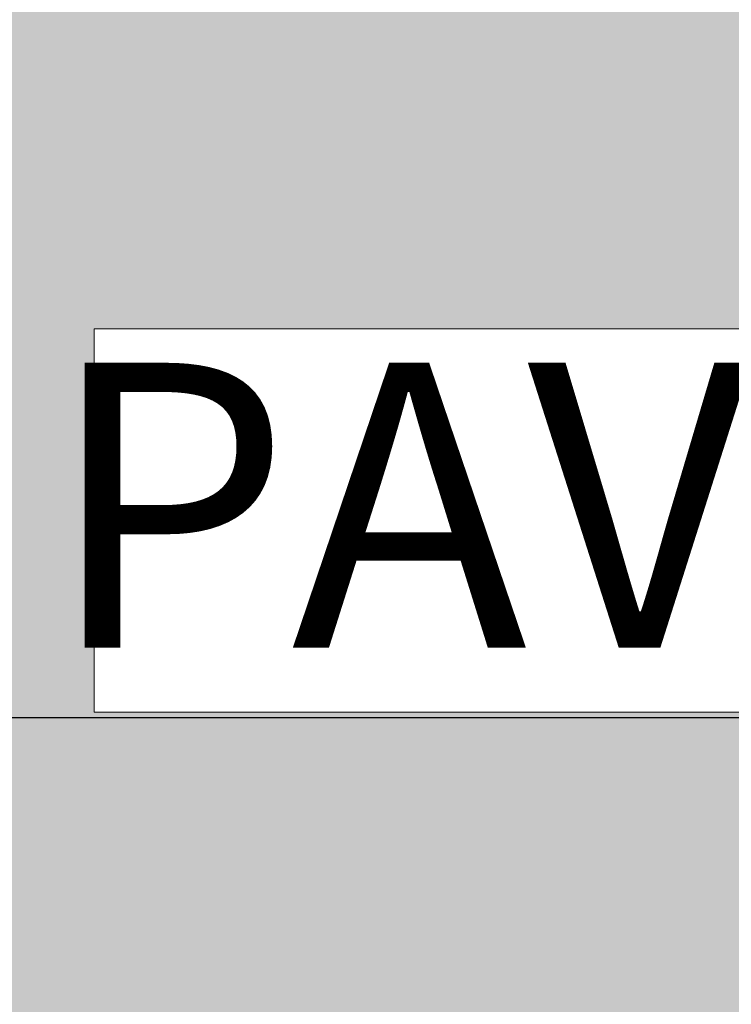
# Model space of a CAD drawing. Units: inches. Extents: x 459864 to 460310, y 324185 to 324787.
# Tile 42 of 112: x 460079 to 460094, y 324221 to 324242. Entities that reach past the tile are written whole.
import ezdxf

# ---------------------------------------------------------------- set-up
doc = ezdxf.new("R2010")
doc.units = ezdxf.units.IN
for name, color, linetype, lineweight in [('A-ANNO-DIMS', 2, 'Continuous', 18), ('L-HRDS', 9, 'Continuous', 18), ('L-SITE-PATT', 252, 'Continuous', 13)]:
    doc.layers.add(name, color=color, linetype=linetype, lineweight=lineweight)
doc.styles.get("Standard").update_dxf_attribs({"font": 'arial.ttf'})
doc.dimstyles.new('ISO-25', dxfattribs={"dimtxt": 6, "dimasz": 2.5, "dimexe": 1.25, "dimexo": 0.625, "dimtad": 1, "dimdec": 1, "dimlunit": 3, "dimtxsty": 'Standard', "dimcen": 2.5, "dimadec": 0, "dimazin": 0, "dimtfac": 1, "dimtdec": 1, "dimtmove": 0, "dimatfit": 3, "dimfxl": 1, "dimarcsym": 0})

# ---------------------------------------------------------------- blocks, each defined once
blk = doc.blocks.new('*D36')
at = {"layer": 'A-ANNO-DIMS', "color": 0, "lineweight": -2, "transparency": 16777216}
for p, q in [((460063.861, 324228.483), (460063.861, 324226.056)), ((460075.876, 324228.483), (460075.876, 324226.056)), ((460066.361, 324227.306), (460073.376, 324227.306)), ((460075.876, 324227.306), (460126.021, 324227.306))]:
    blk.add_line(p, q, dxfattribs=at)
at = {"layer": 'A-ANNO-DIMS', "color": 0, "transparency": 16777216}
for points in [[(460066.361, 324227.722), (460066.361, 324226.889), (460063.861, 324227.306)], [(460073.376, 324227.722), (460073.376, 324226.889), (460075.876, 324227.306)]]:
    blk.add_solid(points, dxfattribs=at)
at = {"layer": 'Defpoints', "color": 0, "transparency": 16777216}
for p in [(460063.861, 324229.108), (460075.876, 324229.108), (460075.876, 324227.306)]:
    blk.add_point(p, dxfattribs=at)
at = {"layer": 'A-ANNO-DIMS', "color": 0, "transparency": 16777216, "insert": (460102.199, 324230.994), "char_height": 6, "attachment_point": 5}
blk.add_mtext('PAVER 1\'-0"', dxfattribs=at)

msp = doc.modelspace()

# ---------------------------------------------------------------- hatches: boundary and pattern name
at = {"layer": 'L-SITE-PATT'}
h = msp.add_hatch(dxfattribs=at)
h.set_pattern_fill('DOTS', color=256)
h.paths.add_polyline_path([(460269.804, 324283.483), (460247.115, 324283.483), (460121.929, 324283.483), (460121.929, 324252.473), (460117.429, 324252.473), (460110.124, 324252.473), (460110.124, 324243.287), (460080.83, 324243.287), (460080.83, 324252.473), (460061.115, 324252.473), (460061.115, 324251.882), (460077.909, 324251.882), (460077.909, 324199.483), (460080.83, 324199.483), (460080.83, 324207.553), (460110.124, 324207.553), (460110.124, 324199.483), (460110.813, 324199.483), (460262.115, 324199.483), (460269.804, 324199.483)], flags=17)
edge = h.paths.add_edge_path(flags=0)
edge.add_ellipse((460222.59, 324263.813), major_axis=(-8.485, 8.485), ratio=1, start_angle=405, end_angle=495, ccw=False)
edge.add_line((460214.821, 324254.66), (460214.832, 324254.666))
edge.add_ellipse((460222.59, 324263.813), major_axis=(-8.485, 8.485), ratio=1, start_angle=405, end_angle=495, ccw=False)
edge.add_line((460210.759, 324261.781), (460210.768, 324261.787))
edge.add_ellipse((460222.59, 324263.813), major_axis=(-8.485, 8.485), ratio=1, start_angle=405, end_angle=495, ccw=False)
edge.add_ellipse((460222.59, 324263.813), major_axis=(-8.485, 8.485), ratio=1, start_angle=392.754, end_angle=405, ccw=False)
edge.add_ellipse((460222.59, 324263.813), major_axis=(-8.485, 8.485), ratio=1, start_angle=380.9347, end_angle=392.754, ccw=False)
edge.add_line((460211.337, 324267.985), (460211.34, 324267.985))
edge.add_ellipse((460222.59, 324263.813), major_axis=(-8.485, 8.485), ratio=1, start_angle=380.9347, end_angle=392.754, ccw=False)
edge.add_ellipse((460222.59, 324263.813), major_axis=(-8.485, 8.485), ratio=1, start_angle=347.9015, end_angle=380.9347, ccw=False)
edge.add_ellipse((460222.59, 324263.813), major_axis=(-8.485, 8.485), ratio=1, start_angle=327.0619, end_angle=347.9015, ccw=False)
edge.add_ellipse((460222.59, 324263.813), major_axis=(-8.485, 8.485), ratio=1, start_angle=278.3246, end_angle=327.0619, ccw=False)
edge.add_line((460225.158, 324275.536), (460225.158, 324275.535))
edge.add_ellipse((460222.59, 324263.813), major_axis=(-8.485, 8.485), ratio=1, start_angle=278.3246, end_angle=327.0619, ccw=False)
edge.add_ellipse((460222.59, 324263.813), major_axis=(-8.485, 8.485), ratio=1, start_angle=260.6436, end_angle=278.3246, ccw=False)
edge.add_ellipse((460222.59, 324263.813), major_axis=(-8.485, 8.485), ratio=1, start_angle=225, end_angle=260.6436, ccw=False)
edge.add_line((460234.509, 324265.243), (460234.501, 324265.239))
edge.add_ellipse((460222.59, 324263.813), major_axis=(-8.485, 8.485), ratio=1, start_angle=225, end_angle=260.6436, ccw=False)
edge.add_ellipse((460222.59, 324263.813), major_axis=(-8.485, 8.485), ratio=1, start_angle=495, end_angle=585, ccw=False)
edge.add_line((460234.437, 324261.861), (460234.424, 324261.858))
edge.add_ellipse((460222.59, 324263.813), major_axis=(-8.485, 8.485), ratio=1, start_angle=495, end_angle=585, ccw=False)
edge.add_line((460227.95, 324253.067), (460227.946, 324253.083))
edge.add_ellipse((460222.59, 324263.813), major_axis=(-8.485, 8.485), ratio=1, start_angle=495, end_angle=585, ccw=False)
edge.add_line((460226.223, 324252.369), (460226.211, 324252.38))
edge.add_ellipse((460222.59, 324263.813), major_axis=(-8.485, 8.485), ratio=1, start_angle=495, end_angle=585, ccw=False)
h.paths.add_polyline_path([(460219.651, 324254.347), (460218.461, 324253.545), (460218.275, 324254.789), (460219.642, 324256.542), (460219.625, 324260.848), (460216.11, 324257.333), (460214.35, 324256.978), (460215.416, 324259.356), (460212.524, 324258.496), (460213.137, 324259.93), (460218.507, 324263.813), (460222.59, 324263.813), (460222.59, 324267.807), (460218.176, 324272.212), (460219.026, 324274.639), (460222.59, 324272.811), (460222.59, 324275.423), (460223.057, 324274.825), (460222.675, 324273.492), (460225.912, 324267.135), (460219.625, 324260.848)], flags=0)
edge = h.paths.add_edge_path(flags=0)
edge.add_ellipse((460194.576, 324264.046), major_axis=(-8.485, 8.485), ratio=1, start_angle=495, end_angle=585, ccw=False)
edge.add_line((460199.936, 324253.3), (460199.932, 324253.316))
edge.add_ellipse((460194.576, 324264.046), major_axis=(-8.485, 8.485), ratio=1, start_angle=495, end_angle=585, ccw=False)
edge.add_line((460198.208, 324252.603), (460198.196, 324252.613))
edge.add_ellipse((460194.576, 324264.046), major_axis=(-8.485, 8.485), ratio=1, start_angle=495, end_angle=585, ccw=False)
edge.add_ellipse((460194.576, 324264.046), major_axis=(-8.485, 8.485), ratio=1, start_angle=405, end_angle=495, ccw=False)
edge.add_line((460186.806, 324254.893), (460186.817, 324254.899))
edge.add_ellipse((460194.576, 324264.046), major_axis=(-8.485, 8.485), ratio=1, start_angle=405, end_angle=495, ccw=False)
edge.add_line((460182.744, 324262.014), (460182.753, 324262.02))
edge.add_ellipse((460194.576, 324264.046), major_axis=(-8.485, 8.485), ratio=1, start_angle=405, end_angle=495, ccw=False)
edge.add_ellipse((460194.576, 324264.046), major_axis=(-8.485, 8.485), ratio=1, start_angle=392.754, end_angle=405, ccw=False)
edge.add_ellipse((460194.576, 324264.046), major_axis=(-8.485, 8.485), ratio=1, start_angle=380.9347, end_angle=392.754, ccw=False)
edge.add_line((460183.323, 324268.218), (460183.326, 324268.218))
edge.add_ellipse((460194.576, 324264.046), major_axis=(-8.485, 8.485), ratio=1, start_angle=380.9347, end_angle=392.754, ccw=False)
edge.add_ellipse((460194.576, 324264.046), major_axis=(-8.485, 8.485), ratio=1, start_angle=347.9015, end_angle=380.9347, ccw=False)
edge.add_ellipse((460194.576, 324264.046), major_axis=(-8.485, 8.485), ratio=1, start_angle=327.0619, end_angle=347.9015, ccw=False)
edge.add_ellipse((460194.576, 324264.046), major_axis=(-8.485, 8.485), ratio=1, start_angle=278.3246, end_angle=327.0619, ccw=False)
edge.add_line((460197.144, 324275.769), (460197.143, 324275.768))
edge.add_ellipse((460194.576, 324264.046), major_axis=(-8.485, 8.485), ratio=1, start_angle=278.3246, end_angle=327.0619, ccw=False)
edge.add_ellipse((460194.576, 324264.046), major_axis=(-8.485, 8.485), ratio=1, start_angle=260.6436, end_angle=278.3246, ccw=False)
edge.add_ellipse((460194.576, 324264.046), major_axis=(-8.485, 8.485), ratio=1, start_angle=225, end_angle=260.6436, ccw=False)
edge.add_line((460206.494, 324265.476), (460206.487, 324265.473))
edge.add_ellipse((460194.576, 324264.046), major_axis=(-8.485, 8.485), ratio=1, start_angle=225, end_angle=260.6436, ccw=False)
edge.add_ellipse((460194.576, 324264.046), major_axis=(-8.485, 8.485), ratio=1, start_angle=495, end_angle=585, ccw=False)
edge.add_line((460206.422, 324262.094), (460206.409, 324262.091))
h.paths.add_polyline_path([(460191.61, 324261.081), (460191.637, 324254.58), (460190.447, 324253.778), (460190.261, 324255.023), (460191.628, 324256.775), (460191.61, 324261.081), (460188.096, 324257.566), (460186.335, 324257.211), (460187.402, 324259.589), (460184.509, 324258.729), (460185.123, 324260.163), (460190.493, 324264.046), (460194.576, 324264.046), (460194.576, 324268.04), (460190.161, 324272.446), (460191.011, 324274.872), (460194.576, 324273.044), (460194.576, 324275.657), (460195.043, 324275.058), (460194.661, 324273.725), (460197.897, 324267.368)], flags=0)
edge = h.paths.add_edge_path(flags=0)
edge.add_ellipse((460252.912, 324263.578), major_axis=(-8.485, 8.485), ratio=1, start_angle=405, end_angle=495, ccw=False)
edge.add_line((460241.081, 324261.545), (460241.089, 324261.551))
edge.add_ellipse((460252.912, 324263.578), major_axis=(-8.485, 8.485), ratio=1, start_angle=405, end_angle=495, ccw=False)
edge.add_ellipse((460252.912, 324263.578), major_axis=(-8.485, 8.485), ratio=1, start_angle=392.754, end_angle=405, ccw=False)
edge.add_ellipse((460252.912, 324263.578), major_axis=(-8.485, 8.485), ratio=1, start_angle=380.9347, end_angle=392.754, ccw=False)
edge.add_line((460241.659, 324267.749), (460241.662, 324267.749))
edge.add_ellipse((460252.912, 324263.578), major_axis=(-8.485, 8.485), ratio=1, start_angle=380.9347, end_angle=392.754, ccw=False)
edge.add_ellipse((460252.912, 324263.578), major_axis=(-8.485, 8.485), ratio=1, start_angle=347.9015, end_angle=380.9347, ccw=False)
edge.add_ellipse((460252.912, 324263.578), major_axis=(-8.485, 8.485), ratio=1, start_angle=327.0619, end_angle=347.9015, ccw=False)
edge.add_ellipse((460252.912, 324263.578), major_axis=(-8.485, 8.485), ratio=1, start_angle=278.3246, end_angle=327.0619, ccw=False)
edge.add_line((460255.48, 324275.3), (460255.479, 324275.299))
edge.add_ellipse((460252.912, 324263.578), major_axis=(-8.485, 8.485), ratio=1, start_angle=278.3246, end_angle=327.0619, ccw=False)
edge.add_ellipse((460252.912, 324263.578), major_axis=(-8.485, 8.485), ratio=1, start_angle=260.6436, end_angle=278.3246, ccw=False)
edge.add_ellipse((460252.912, 324263.578), major_axis=(-8.485, 8.485), ratio=1, start_angle=225, end_angle=260.6436, ccw=False)
edge.add_line((460264.83, 324265.007), (460264.823, 324265.004))
edge.add_ellipse((460252.912, 324263.578), major_axis=(-8.485, 8.485), ratio=1, start_angle=225, end_angle=260.6436, ccw=False)
edge.add_ellipse((460252.912, 324263.578), major_axis=(-8.485, 8.485), ratio=1, start_angle=495, end_angle=585, ccw=False)
edge.add_line((460264.758, 324261.626), (460264.745, 324261.622))
edge.add_ellipse((460252.912, 324263.578), major_axis=(-8.485, 8.485), ratio=1, start_angle=495, end_angle=585, ccw=False)
edge.add_line((460258.272, 324252.832), (460258.268, 324252.848))
edge.add_ellipse((460252.912, 324263.578), major_axis=(-8.485, 8.485), ratio=1, start_angle=495, end_angle=585, ccw=False)
edge.add_line((460256.545, 324252.134), (460256.533, 324252.144))
edge.add_ellipse((460252.912, 324263.578), major_axis=(-8.485, 8.485), ratio=1, start_angle=495, end_angle=585, ccw=False)
edge.add_ellipse((460252.912, 324263.578), major_axis=(-8.485, 8.485), ratio=1, start_angle=405, end_angle=495, ccw=False)
edge.add_line((460245.143, 324254.424), (460245.153, 324254.43))
h.paths.add_polyline_path([(460244.672, 324256.742), (460245.738, 324259.12), (460242.846, 324258.26), (460243.459, 324259.694), (460248.829, 324263.578), (460252.912, 324263.578), (460252.912, 324267.571), (460248.497, 324271.977), (460249.348, 324274.403), (460252.912, 324272.576), (460252.912, 324275.188), (460253.379, 324274.589), (460252.997, 324273.257), (460256.233, 324266.899), (460249.946, 324260.612), (460249.973, 324254.111), (460248.783, 324253.309), (460248.597, 324254.554), (460249.964, 324256.306), (460249.946, 324260.612), (460246.432, 324257.097)], flags=0)
edge = h.paths.add_edge_path(flags=0)
edge.add_ellipse((460167.439, 324262.833), major_axis=(-8.485, 8.485), ratio=1, start_angle=495, end_angle=585, ccw=False)
edge.add_line((460172.799, 324252.087), (460172.795, 324252.103))
edge.add_ellipse((460167.439, 324262.833), major_axis=(-8.485, 8.485), ratio=1, start_angle=495, end_angle=585, ccw=False)
edge.add_line((460171.071, 324251.389), (460171.059, 324251.399))
edge.add_ellipse((460167.439, 324262.833), major_axis=(-8.485, 8.485), ratio=1, start_angle=495, end_angle=585, ccw=False)
edge.add_ellipse((460167.439, 324262.833), major_axis=(-8.485, 8.485), ratio=1, start_angle=405, end_angle=495, ccw=False)
edge.add_line((460159.669, 324253.679), (460159.68, 324253.685))
edge.add_ellipse((460167.439, 324262.833), major_axis=(-8.485, 8.485), ratio=1, start_angle=405, end_angle=495, ccw=False)
edge.add_line((460155.607, 324260.8), (460155.616, 324260.806))
edge.add_ellipse((460167.439, 324262.833), major_axis=(-8.485, 8.485), ratio=1, start_angle=405, end_angle=495, ccw=False)
edge.add_ellipse((460167.439, 324262.833), major_axis=(-8.485, 8.485), ratio=1, start_angle=392.754, end_angle=405, ccw=False)
edge.add_ellipse((460167.439, 324262.833), major_axis=(-8.485, 8.485), ratio=1, start_angle=380.9347, end_angle=392.754, ccw=False)
edge.add_line((460156.185, 324267.005), (460156.189, 324267.005))
edge.add_ellipse((460167.439, 324262.833), major_axis=(-8.485, 8.485), ratio=1, start_angle=380.9347, end_angle=392.754, ccw=False)
edge.add_ellipse((460167.439, 324262.833), major_axis=(-8.485, 8.485), ratio=1, start_angle=347.9015, end_angle=380.9347, ccw=False)
edge.add_ellipse((460167.439, 324262.833), major_axis=(-8.485, 8.485), ratio=1, start_angle=327.0619, end_angle=347.9015, ccw=False)
edge.add_ellipse((460167.439, 324262.833), major_axis=(-8.485, 8.485), ratio=1, start_angle=278.3246, end_angle=327.0619, ccw=False)
edge.add_line((460170.007, 324274.556), (460170.006, 324274.554))
edge.add_ellipse((460167.439, 324262.833), major_axis=(-8.485, 8.485), ratio=1, start_angle=278.3246, end_angle=327.0619, ccw=False)
edge.add_ellipse((460167.439, 324262.833), major_axis=(-8.485, 8.485), ratio=1, start_angle=260.6436, end_angle=278.3246, ccw=False)
edge.add_ellipse((460167.439, 324262.833), major_axis=(-8.485, 8.485), ratio=1, start_angle=225, end_angle=260.6436, ccw=False)
edge.add_line((460179.357, 324264.262), (460179.35, 324264.259))
edge.add_ellipse((460167.439, 324262.833), major_axis=(-8.485, 8.485), ratio=1, start_angle=225, end_angle=260.6436, ccw=False)
edge.add_ellipse((460167.439, 324262.833), major_axis=(-8.485, 8.485), ratio=1, start_angle=495, end_angle=585, ccw=False)
edge.add_line((460179.285, 324260.881), (460179.272, 324260.877))
h.paths.add_polyline_path([(460164.473, 324259.867), (460164.5, 324253.366), (460163.31, 324252.565), (460163.124, 324253.809), (460164.491, 324255.561), (460164.473, 324259.867), (460160.958, 324256.353), (460159.198, 324255.998), (460160.265, 324258.375), (460157.372, 324257.515), (460157.986, 324258.949), (460163.356, 324262.833), (460167.439, 324262.833), (460167.439, 324266.826), (460163.024, 324271.232), (460163.874, 324273.659), (460167.439, 324271.831), (460167.439, 324274.443), (460167.905, 324273.844), (460167.524, 324272.512), (460170.76, 324266.154)], flags=0)
edge = h.paths.add_edge_path(flags=0)
edge.add_ellipse((460140.758, 324262.37), major_axis=(-8.485, 8.485), ratio=1, start_angle=495, end_angle=585, ccw=False)
edge.add_line((460146.118, 324251.624), (460146.114, 324251.639))
edge.add_ellipse((460140.758, 324262.37), major_axis=(-8.485, 8.485), ratio=1, start_angle=495, end_angle=585, ccw=False)
edge.add_line((460144.391, 324250.926), (460144.379, 324250.936))
edge.add_ellipse((460140.758, 324262.37), major_axis=(-8.485, 8.485), ratio=1, start_angle=495, end_angle=585, ccw=False)
edge.add_ellipse((460140.758, 324262.37), major_axis=(-8.485, 8.485), ratio=1, start_angle=405, end_angle=495, ccw=False)
edge.add_line((460132.989, 324253.216), (460132.999, 324253.222))
edge.add_ellipse((460140.758, 324262.37), major_axis=(-8.485, 8.485), ratio=1, start_angle=405, end_angle=495, ccw=False)
edge.add_line((460128.927, 324260.337), (460128.935, 324260.343))
edge.add_ellipse((460140.758, 324262.37), major_axis=(-8.485, 8.485), ratio=1, start_angle=405, end_angle=495, ccw=False)
edge.add_ellipse((460140.758, 324262.37), major_axis=(-8.485, 8.485), ratio=1, start_angle=392.754, end_angle=405, ccw=False)
edge.add_ellipse((460140.758, 324262.37), major_axis=(-8.485, 8.485), ratio=1, start_angle=380.9347, end_angle=392.754, ccw=False)
edge.add_line((460129.505, 324266.541), (460129.508, 324266.541))
edge.add_ellipse((460140.758, 324262.37), major_axis=(-8.485, 8.485), ratio=1, start_angle=380.9347, end_angle=392.754, ccw=False)
edge.add_ellipse((460140.758, 324262.37), major_axis=(-8.485, 8.485), ratio=1, start_angle=347.9015, end_angle=380.9347, ccw=False)
edge.add_ellipse((460140.758, 324262.37), major_axis=(-8.485, 8.485), ratio=1, start_angle=327.0619, end_angle=347.9015, ccw=False)
edge.add_ellipse((460140.758, 324262.37), major_axis=(-8.485, 8.485), ratio=1, start_angle=278.3246, end_angle=327.0619, ccw=False)
edge.add_line((460143.326, 324274.092), (460143.325, 324274.091))
edge.add_ellipse((460140.758, 324262.37), major_axis=(-8.485, 8.485), ratio=1, start_angle=278.3246, end_angle=327.0619, ccw=False)
edge.add_ellipse((460140.758, 324262.37), major_axis=(-8.485, 8.485), ratio=1, start_angle=260.6436, end_angle=278.3246, ccw=False)
edge.add_ellipse((460140.758, 324262.37), major_axis=(-8.485, 8.485), ratio=1, start_angle=225, end_angle=260.6436, ccw=False)
edge.add_line((460152.677, 324263.799), (460152.669, 324263.796))
edge.add_ellipse((460140.758, 324262.37), major_axis=(-8.485, 8.485), ratio=1, start_angle=225, end_angle=260.6436, ccw=False)
edge.add_ellipse((460140.758, 324262.37), major_axis=(-8.485, 8.485), ratio=1, start_angle=495, end_angle=585, ccw=False)
edge.add_line((460152.604, 324260.418), (460152.592, 324260.414))
h.paths.add_polyline_path([(460137.792, 324259.404), (460137.819, 324252.903), (460136.629, 324252.101), (460136.443, 324253.346), (460137.81, 324255.098), (460137.792, 324259.404), (460134.278, 324255.889), (460132.518, 324255.534), (460133.584, 324257.912), (460130.692, 324257.052), (460131.305, 324258.486), (460136.675, 324262.37), (460140.758, 324262.37), (460140.758, 324266.363), (460136.343, 324270.769), (460137.194, 324273.195), (460140.758, 324271.367), (460140.758, 324273.98), (460141.225, 324273.381), (460140.843, 324272.049), (460144.079, 324265.691)], flags=0)
h.paths.add_polyline_path([(460110.124, 324227.414), (460080.83, 324227.414), (460080.83, 324235.484), (460110.124, 324235.484)], flags=16)
h.paths.add_polyline_path([(460110.124, 324220.797), (460110.124, 324212.727), (460080.83, 324212.727), (460080.83, 324220.797)], flags=16)
h.paths.add_polyline_path([(460269.804, 324283.483), (460247.115, 324283.483), (460121.929, 324283.483), (460121.929, 324252.473), (460117.429, 324252.473), (460110.124, 324252.473), (460110.124, 324243.287), (460080.83, 324243.287), (460080.83, 324252.473), (460061.115, 324252.473), (460061.115, 324251.882), (460077.909, 324251.882), (460077.909, 324199.483), (460080.83, 324199.483), (460080.83, 324207.553), (460110.124, 324207.553), (460110.124, 324199.483), (460262.115, 324199.483), (460269.804, 324199.483)], flags=17)
h.paths.add_polyline_path([(460219.651, 324254.347), (460218.461, 324253.545), (460218.275, 324254.789), (460219.642, 324256.542), (460219.625, 324260.848), (460216.11, 324257.333), (460214.35, 324256.978), (460215.416, 324259.356), (460212.524, 324258.496), (460213.137, 324259.93), (460218.507, 324263.813), (460222.59, 324263.813), (460220.18, 324266.223), (460215.461, 324265.308), (460211.835, 324266.137), (460216.247, 324267.985), (460218.418, 324267.985), (460222.59, 324263.813), (460222.59, 324267.807), (460218.176, 324272.212), (460219.026, 324274.639), (460222.59, 324272.811), (460222.59, 324275.423), (460223.057, 324274.825), (460222.675, 324273.492), (460225.912, 324267.135), (460222.59, 324263.813), (460231.383, 324263.813), (460228.485, 324262.488), (460224.425, 324261.978), (460228.68, 324257.724), (460228.966, 324254.791), (460227.142, 324256.537), (460227.542, 324254.819), (460227.333, 324253.614), (460222.59, 324259.985), (460222.59, 324255.497), (460221.377, 324256.541), (460220.576, 324261.799), (460219.625, 324260.848)], flags=0)
h.paths.add_polyline_path([(460199.127, 324256.77), (460199.528, 324255.052), (460199.319, 324253.848), (460194.576, 324260.218), (460194.576, 324255.73), (460193.363, 324256.774), (460192.561, 324262.032), (460191.61, 324261.081), (460191.637, 324254.58), (460190.447, 324253.778), (460190.261, 324255.023), (460191.628, 324256.775), (460191.61, 324261.081), (460188.096, 324257.566), (460186.335, 324257.211), (460187.402, 324259.589), (460184.509, 324258.729), (460185.123, 324260.163), (460190.493, 324264.046), (460194.576, 324264.046), (460192.166, 324266.456), (460187.446, 324265.541), (460183.82, 324266.37), (460188.232, 324268.218), (460190.404, 324268.218), (460194.576, 324264.046), (460194.576, 324268.04), (460190.161, 324272.446), (460191.011, 324274.872), (460194.576, 324273.044), (460194.576, 324275.657), (460195.043, 324275.058), (460194.661, 324273.725), (460197.897, 324267.368), (460194.576, 324264.046), (460203.368, 324264.046), (460200.47, 324262.721), (460196.411, 324262.212), (460200.665, 324257.957), (460200.951, 324255.024)], flags=0)
h.paths.add_polyline_path([(460244.672, 324256.742), (460245.738, 324259.12), (460242.846, 324258.26), (460243.459, 324259.694), (460248.829, 324263.578), (460252.912, 324263.578), (460250.502, 324265.987), (460245.783, 324265.072), (460242.156, 324265.901), (460246.568, 324267.749), (460248.74, 324267.749), (460252.912, 324263.578), (460252.912, 324267.571), (460248.497, 324271.977), (460249.348, 324274.403), (460252.912, 324272.576), (460252.912, 324275.188), (460253.379, 324274.589), (460252.997, 324273.257), (460256.233, 324266.899), (460252.912, 324263.578), (460261.705, 324263.578), (460258.806, 324262.252), (460254.747, 324261.743), (460259.002, 324257.488), (460259.288, 324254.555), (460257.463, 324256.301), (460257.864, 324254.583), (460257.655, 324253.379), (460252.912, 324259.749), (460252.912, 324255.261), (460251.699, 324256.305), (460250.897, 324261.563), (460249.946, 324260.612), (460249.973, 324254.111), (460248.783, 324253.309), (460248.597, 324254.554), (460249.964, 324256.306), (460249.946, 324260.612), (460246.432, 324257.097)], flags=0)
h.paths.add_polyline_path([(460173.528, 324256.743), (460173.814, 324253.811), (460171.99, 324255.556), (460172.39, 324253.838), (460172.182, 324252.634), (460167.439, 324259.004), (460167.439, 324254.516), (460166.226, 324255.56), (460165.424, 324260.818), (460164.473, 324259.867), (460164.5, 324253.366), (460163.31, 324252.565), (460163.124, 324253.809), (460164.491, 324255.561), (460164.473, 324259.867), (460160.958, 324256.353), (460159.198, 324255.998), (460160.265, 324258.375), (460157.372, 324257.515), (460157.986, 324258.949), (460163.356, 324262.833), (460167.439, 324262.833), (460165.029, 324265.243), (460160.309, 324264.327), (460156.683, 324265.156), (460161.095, 324267.005), (460163.267, 324267.005), (460167.439, 324262.833), (460167.439, 324266.826), (460163.024, 324271.232), (460163.874, 324273.659), (460167.439, 324271.831), (460167.439, 324274.443), (460167.905, 324273.844), (460167.524, 324272.512), (460170.76, 324266.154), (460167.439, 324262.833), (460176.231, 324262.833), (460173.333, 324261.507), (460169.274, 324260.998)], flags=0)
h.paths.add_polyline_path([(460146.848, 324256.28), (460147.134, 324253.347), (460145.31, 324255.093), (460145.71, 324253.375), (460145.501, 324252.171), (460140.758, 324258.541), (460140.758, 324254.053), (460139.545, 324255.097), (460138.744, 324260.355), (460137.792, 324259.404), (460137.819, 324252.903), (460136.629, 324252.101), (460136.443, 324253.346), (460137.81, 324255.098), (460137.792, 324259.404), (460134.278, 324255.889), (460132.518, 324255.534), (460133.584, 324257.912), (460130.692, 324257.052), (460131.305, 324258.486), (460136.675, 324262.37), (460140.758, 324262.37), (460138.348, 324264.779), (460133.629, 324263.864), (460130.002, 324264.693), (460134.414, 324266.541), (460136.586, 324266.541), (460140.758, 324262.37), (460140.758, 324266.363), (460136.343, 324270.769), (460137.194, 324273.195), (460140.758, 324271.367), (460140.758, 324273.98), (460141.225, 324273.381), (460140.843, 324272.049), (460144.079, 324265.691), (460140.758, 324262.37), (460149.551, 324262.37), (460146.653, 324261.044), (460142.593, 324260.535)], flags=0)
edge = h.paths.add_edge_path()
edge.add_line((460269.804, 324272.549), (460260.881, 324272.549))
edge.add_ellipse((460252.912, 324263.578), major_axis=(-8.485, 8.485), ratio=1, start_angle=260.6436, end_angle=273.3846, ccw=False)
edge.add_line((460262.283, 324271.092), (460262.261, 324271.091))
edge.add_ellipse((460252.912, 324263.578), major_axis=(-8.485, 8.485), ratio=1, start_angle=260.6436, end_angle=273.3846, ccw=False)
edge.add_ellipse((460252.912, 324263.578), major_axis=(-8.485, 8.485), ratio=1, start_angle=225, end_angle=260.6436, ccw=False)
edge.add_line((460263.609, 324269.063), (460263.572, 324269.058))
edge.add_ellipse((460252.912, 324263.578), major_axis=(-8.485, 8.485), ratio=1, start_angle=225, end_angle=260.6436, ccw=False)
edge.add_line((460264.615, 324266.306), (460264.585, 324266.305))
edge.add_ellipse((460252.912, 324263.578), major_axis=(-8.485, 8.485), ratio=1, start_angle=225, end_angle=260.6436, ccw=False)
edge.add_line((460264.83, 324265.007), (460264.823, 324265.004))
edge.add_ellipse((460252.912, 324263.578), major_axis=(-8.485, 8.485), ratio=1, start_angle=225, end_angle=260.6436, ccw=False)
edge.add_ellipse((460252.912, 324263.578), major_axis=(-8.485, 8.485), ratio=1, start_angle=495, end_angle=585, ccw=False)
edge.add_line((460264.758, 324261.626), (460264.745, 324261.622))
edge.add_ellipse((460252.912, 324263.578), major_axis=(-8.485, 8.485), ratio=1, start_angle=495, end_angle=585, ccw=False)
edge.add_line((460263.442, 324257.739), (460263.389, 324257.779))
edge.add_ellipse((460252.912, 324263.578), major_axis=(-8.485, 8.485), ratio=1, start_angle=495, end_angle=585, ccw=False)
edge.add_line((460258.128, 324252.744), (460258.102, 324252.779))
edge.add_ellipse((460252.912, 324263.578), major_axis=(-8.485, 8.485), ratio=1, start_angle=495, end_angle=585, ccw=False)
edge.add_line((460256.545, 324252.134), (460256.533, 324252.144))
edge.add_ellipse((460252.912, 324263.578), major_axis=(-8.485, 8.485), ratio=1, start_angle=495, end_angle=585, ccw=False)
edge.add_ellipse((460252.912, 324263.578), major_axis=(-8.485, 8.485), ratio=1, start_angle=405, end_angle=495, ccw=False)
edge.add_line((460250.594, 324251.78), (460250.605, 324251.82))
edge.add_ellipse((460252.912, 324263.578), major_axis=(-8.485, 8.485), ratio=1, start_angle=405, end_angle=495, ccw=False)
edge.add_line((460245.143, 324254.424), (460245.153, 324254.43))
edge.add_ellipse((460252.912, 324263.578), major_axis=(-8.485, 8.485), ratio=1, start_angle=405, end_angle=495, ccw=False)
edge.add_line((460243.525, 324256.059), (460243.56, 324256.091))
edge.add_ellipse((460252.912, 324263.578), major_axis=(-8.485, 8.485), ratio=1, start_angle=405, end_angle=495, ccw=False)
edge.add_line((460241.44, 324259.893), (460241.522, 324259.896))
edge.add_ellipse((460252.912, 324263.578), major_axis=(-8.485, 8.485), ratio=1, start_angle=405, end_angle=495, ccw=False)
edge.add_line((460241.081, 324261.545), (460241.089, 324261.551))
edge.add_ellipse((460252.912, 324263.578), major_axis=(-8.485, 8.485), ratio=1, start_angle=405, end_angle=495, ccw=False)
edge.add_ellipse((460252.912, 324263.578), major_axis=(-8.485, 8.485), ratio=1, start_angle=392.754, end_angle=405, ccw=False)
edge.add_line((460241.05, 324265.438), (460241.063, 324265.443))
edge.add_ellipse((460252.912, 324263.578), major_axis=(-8.485, 8.485), ratio=1, start_angle=392.754, end_angle=405, ccw=False)
edge.add_ellipse((460252.912, 324263.578), major_axis=(-8.485, 8.485), ratio=1, start_angle=380.9347, end_angle=392.754, ccw=False)
edge.add_line((460241.452, 324267.176), (460241.469, 324267.171))
edge.add_ellipse((460252.912, 324263.578), major_axis=(-8.485, 8.485), ratio=1, start_angle=380.9347, end_angle=392.754, ccw=False)
edge.add_line((460241.659, 324267.749), (460241.662, 324267.749))
edge.add_ellipse((460252.912, 324263.578), major_axis=(-8.485, 8.485), ratio=1, start_angle=380.9347, end_angle=392.754, ccw=False)
edge.add_ellipse((460252.912, 324263.578), major_axis=(-8.485, 8.485), ratio=1, start_angle=356.6154, end_angle=380.9347, ccw=False)
edge.add_line((460244.88, 324272.488), (460244.713, 324272.549))
edge.add_line((460244.713, 324272.549), (460230.817, 324272.549))
edge.add_ellipse((460222.59, 324263.813), major_axis=(-8.485, 8.485), ratio=1, start_angle=260.6436, end_angle=271.7178, ccw=False)
edge.add_ellipse((460222.59, 324263.813), major_axis=(-8.485, 8.485), ratio=1, start_angle=225, end_angle=260.6436, ccw=False)
edge.add_line((460233.287, 324269.299), (460233.25, 324269.294))
edge.add_ellipse((460222.59, 324263.813), major_axis=(-8.485, 8.485), ratio=1, start_angle=225, end_angle=260.6436, ccw=False)
edge.add_line((460234.294, 324266.541), (460234.264, 324266.541))
edge.add_ellipse((460222.59, 324263.813), major_axis=(-8.485, 8.485), ratio=1, start_angle=225, end_angle=260.6436, ccw=False)
edge.add_line((460234.509, 324265.243), (460234.501, 324265.239))
edge.add_ellipse((460222.59, 324263.813), major_axis=(-8.485, 8.485), ratio=1, start_angle=225, end_angle=260.6436, ccw=False)
edge.add_ellipse((460222.59, 324263.813), major_axis=(-8.485, 8.485), ratio=1, start_angle=495, end_angle=585, ccw=False)
edge.add_line((460234.437, 324261.861), (460234.424, 324261.858))
edge.add_ellipse((460222.59, 324263.813), major_axis=(-8.485, 8.485), ratio=1, start_angle=495, end_angle=585, ccw=False)
edge.add_line((460233.121, 324257.975), (460233.068, 324258.015))
edge.add_ellipse((460222.59, 324263.813), major_axis=(-8.485, 8.485), ratio=1, start_angle=495, end_angle=585, ccw=False)
edge.add_line((460227.806, 324252.979), (460227.78, 324253.014))
edge.add_ellipse((460222.59, 324263.813), major_axis=(-8.485, 8.485), ratio=1, start_angle=495, end_angle=585, ccw=False)
edge.add_line((460226.223, 324252.369), (460226.211, 324252.38))
edge.add_ellipse((460222.59, 324263.813), major_axis=(-8.485, 8.485), ratio=1, start_angle=495, end_angle=585, ccw=False)
edge.add_ellipse((460222.59, 324263.813), major_axis=(-8.485, 8.485), ratio=1, start_angle=405, end_angle=495, ccw=False)
edge.add_line((460220.272, 324252.016), (460220.283, 324252.055))
edge.add_ellipse((460222.59, 324263.813), major_axis=(-8.485, 8.485), ratio=1, start_angle=405, end_angle=495, ccw=False)
edge.add_line((460214.821, 324254.66), (460214.832, 324254.666))
edge.add_ellipse((460222.59, 324263.813), major_axis=(-8.485, 8.485), ratio=1, start_angle=405, end_angle=495, ccw=False)
edge.add_line((460213.203, 324256.295), (460213.239, 324256.327))
edge.add_ellipse((460222.59, 324263.813), major_axis=(-8.485, 8.485), ratio=1, start_angle=405, end_angle=495, ccw=False)
edge.add_line((460211.118, 324260.128), (460211.201, 324260.131))
edge.add_ellipse((460222.59, 324263.813), major_axis=(-8.485, 8.485), ratio=1, start_angle=405, end_angle=495, ccw=False)
edge.add_line((460210.759, 324261.781), (460210.768, 324261.787))
edge.add_ellipse((460222.59, 324263.813), major_axis=(-8.485, 8.485), ratio=1, start_angle=405, end_angle=495, ccw=False)
edge.add_ellipse((460222.59, 324263.813), major_axis=(-8.485, 8.485), ratio=1, start_angle=392.754, end_angle=405, ccw=False)
edge.add_line((460210.729, 324265.673), (460210.741, 324265.678))
edge.add_ellipse((460222.59, 324263.813), major_axis=(-8.485, 8.485), ratio=1, start_angle=392.754, end_angle=405, ccw=False)
edge.add_ellipse((460222.59, 324263.813), major_axis=(-8.485, 8.485), ratio=1, start_angle=380.9347, end_angle=392.754, ccw=False)
edge.add_line((460211.13, 324267.412), (460211.147, 324267.407))
edge.add_ellipse((460222.59, 324263.813), major_axis=(-8.485, 8.485), ratio=1, start_angle=380.9347, end_angle=392.754, ccw=False)
edge.add_line((460211.337, 324267.985), (460211.34, 324267.985))
edge.add_ellipse((460222.59, 324263.813), major_axis=(-8.485, 8.485), ratio=1, start_angle=380.9347, end_angle=392.754, ccw=False)
edge.add_ellipse((460222.59, 324263.813), major_axis=(-8.485, 8.485), ratio=1, start_angle=358.2822, end_angle=380.9347, ccw=False)
edge.add_line((460213.705, 324271.902), (460213.709, 324271.869))
edge.add_ellipse((460222.59, 324263.813), major_axis=(-8.485, 8.485), ratio=1, start_angle=358.2822, end_angle=380.9347, ccw=False)
edge.add_line((460214.363, 324272.549), (460203.078, 324272.549))
edge.add_line((460203.078, 324272.549), (460203.06, 324272.531))
edge.add_ellipse((460194.576, 324264.046), major_axis=(-8.485, 8.485), ratio=1, start_angle=260.6436, end_angle=270.1168, ccw=False)
edge.add_line((460203.957, 324271.561), (460203.921, 324271.56))
edge.add_ellipse((460194.576, 324264.046), major_axis=(-8.485, 8.485), ratio=1, start_angle=260.6436, end_angle=270.1168, ccw=False)
edge.add_ellipse((460194.576, 324264.046), major_axis=(-8.485, 8.485), ratio=1, start_angle=225, end_angle=260.6436, ccw=False)
edge.add_line((460205.272, 324269.532), (460205.235, 324269.527))
edge.add_ellipse((460194.576, 324264.046), major_axis=(-8.485, 8.485), ratio=1, start_angle=225, end_angle=260.6436, ccw=False)
edge.add_line((460206.279, 324266.774), (460206.249, 324266.774))
edge.add_ellipse((460194.576, 324264.046), major_axis=(-8.485, 8.485), ratio=1, start_angle=225, end_angle=260.6436, ccw=False)
edge.add_line((460206.494, 324265.476), (460206.487, 324265.473))
edge.add_ellipse((460194.576, 324264.046), major_axis=(-8.485, 8.485), ratio=1, start_angle=225, end_angle=260.6436, ccw=False)
edge.add_ellipse((460194.576, 324264.046), major_axis=(-8.485, 8.485), ratio=1, start_angle=495, end_angle=585, ccw=False)
edge.add_line((460206.422, 324262.094), (460206.409, 324262.091))
edge.add_ellipse((460194.576, 324264.046), major_axis=(-8.485, 8.485), ratio=1, start_angle=495, end_angle=585, ccw=False)
edge.add_line((460205.106, 324258.208), (460205.053, 324258.248))
edge.add_ellipse((460194.576, 324264.046), major_axis=(-8.485, 8.485), ratio=1, start_angle=495, end_angle=585, ccw=False)
edge.add_line((460199.792, 324253.212), (460199.766, 324253.248))
edge.add_ellipse((460194.576, 324264.046), major_axis=(-8.485, 8.485), ratio=1, start_angle=495, end_angle=585, ccw=False)
edge.add_line((460198.208, 324252.603), (460198.196, 324252.613))
edge.add_ellipse((460194.576, 324264.046), major_axis=(-8.485, 8.485), ratio=1, start_angle=495, end_angle=585, ccw=False)
edge.add_ellipse((460194.576, 324264.046), major_axis=(-8.485, 8.485), ratio=1, start_angle=405, end_angle=495, ccw=False)
edge.add_line((460192.258, 324252.249), (460192.268, 324252.289))
edge.add_ellipse((460194.576, 324264.046), major_axis=(-8.485, 8.485), ratio=1, start_angle=405, end_angle=495, ccw=False)
edge.add_line((460186.806, 324254.893), (460186.817, 324254.899))
edge.add_ellipse((460194.576, 324264.046), major_axis=(-8.485, 8.485), ratio=1, start_angle=405, end_angle=495, ccw=False)
edge.add_line((460185.188, 324256.528), (460185.224, 324256.56))
edge.add_ellipse((460194.576, 324264.046), major_axis=(-8.485, 8.485), ratio=1, start_angle=405, end_angle=495, ccw=False)
edge.add_line((460183.104, 324260.362), (460183.186, 324260.365))
edge.add_ellipse((460194.576, 324264.046), major_axis=(-8.485, 8.485), ratio=1, start_angle=405, end_angle=495, ccw=False)
edge.add_line((460182.744, 324262.014), (460182.753, 324262.02))
edge.add_ellipse((460194.576, 324264.046), major_axis=(-8.485, 8.485), ratio=1, start_angle=405, end_angle=495, ccw=False)
edge.add_ellipse((460194.576, 324264.046), major_axis=(-8.485, 8.485), ratio=1, start_angle=392.754, end_angle=405, ccw=False)
edge.add_line((460182.714, 324265.906), (460182.726, 324265.912))
edge.add_ellipse((460194.576, 324264.046), major_axis=(-8.485, 8.485), ratio=1, start_angle=392.754, end_angle=405, ccw=False)
edge.add_ellipse((460194.576, 324264.046), major_axis=(-8.485, 8.485), ratio=1, start_angle=380.9347, end_angle=392.754, ccw=False)
edge.add_line((460183.116, 324267.645), (460183.133, 324267.64))
edge.add_ellipse((460194.576, 324264.046), major_axis=(-8.485, 8.485), ratio=1, start_angle=380.9347, end_angle=392.754, ccw=False)
edge.add_line((460183.323, 324268.218), (460183.326, 324268.218))
edge.add_ellipse((460194.576, 324264.046), major_axis=(-8.485, 8.485), ratio=1, start_angle=380.9347, end_angle=392.754, ccw=False)
edge.add_ellipse((460194.576, 324264.046), major_axis=(-8.485, 8.485), ratio=1, start_angle=359.8832, end_angle=380.9347, ccw=False)
edge.add_line((460184.491, 324270.611), (460184.553, 324270.611))
edge.add_ellipse((460194.576, 324264.046), major_axis=(-8.485, 8.485), ratio=1, start_angle=359.8832, end_angle=380.9347, ccw=False)
edge.add_line((460185.346, 324271.76), (460185.379, 324271.728))
edge.add_ellipse((460194.576, 324264.046), major_axis=(-8.485, 8.485), ratio=1, start_angle=359.8832, end_angle=380.9347, ccw=False)
edge.add_line((460185.697, 324272.086), (460185.633, 324272.549))
edge.add_line((460185.633, 324272.549), (460174.683, 324272.549))
edge.add_line((460174.683, 324272.549), (460174.606, 324272.457))
edge.add_ellipse((460167.439, 324262.833), major_axis=(-8.485, 8.485), ratio=1, start_angle=260.6436, end_angle=278.3246, ccw=False)
edge.add_ellipse((460167.439, 324262.833), major_axis=(-8.485, 8.485), ratio=1, start_angle=225, end_angle=260.6436, ccw=False)
edge.add_line((460178.135, 324268.318), (460178.098, 324268.313))
edge.add_ellipse((460167.439, 324262.833), major_axis=(-8.485, 8.485), ratio=1, start_angle=225, end_angle=260.6436, ccw=False)
edge.add_line((460179.142, 324265.561), (460179.112, 324265.56))
edge.add_ellipse((460167.439, 324262.833), major_axis=(-8.485, 8.485), ratio=1, start_angle=225, end_angle=260.6436, ccw=False)
edge.add_line((460179.357, 324264.262), (460179.35, 324264.259))
edge.add_ellipse((460167.439, 324262.833), major_axis=(-8.485, 8.485), ratio=1, start_angle=225, end_angle=260.6436, ccw=False)
edge.add_ellipse((460167.439, 324262.833), major_axis=(-8.485, 8.485), ratio=1, start_angle=495, end_angle=585, ccw=False)
edge.add_line((460179.285, 324260.881), (460179.272, 324260.877))
edge.add_ellipse((460167.439, 324262.833), major_axis=(-8.485, 8.485), ratio=1, start_angle=495, end_angle=585, ccw=False)
edge.add_line((460177.969, 324256.994), (460177.916, 324257.034))
edge.add_ellipse((460167.439, 324262.833), major_axis=(-8.485, 8.485), ratio=1, start_angle=495, end_angle=585, ccw=False)
edge.add_line((460172.655, 324251.999), (460172.629, 324252.034))
edge.add_ellipse((460167.439, 324262.833), major_axis=(-8.485, 8.485), ratio=1, start_angle=495, end_angle=585, ccw=False)
edge.add_line((460171.071, 324251.389), (460171.059, 324251.399))
edge.add_ellipse((460167.439, 324262.833), major_axis=(-8.485, 8.485), ratio=1, start_angle=495, end_angle=585, ccw=False)
edge.add_ellipse((460167.439, 324262.833), major_axis=(-8.485, 8.485), ratio=1, start_angle=405, end_angle=495, ccw=False)
edge.add_line((460165.121, 324251.036), (460165.131, 324251.075))
edge.add_ellipse((460167.439, 324262.833), major_axis=(-8.485, 8.485), ratio=1, start_angle=405, end_angle=495, ccw=False)
edge.add_line((460159.669, 324253.679), (460159.68, 324253.685))
edge.add_ellipse((460167.439, 324262.833), major_axis=(-8.485, 8.485), ratio=1, start_angle=405, end_angle=495, ccw=False)
edge.add_line((460158.051, 324255.314), (460158.087, 324255.347))
edge.add_ellipse((460167.439, 324262.833), major_axis=(-8.485, 8.485), ratio=1, start_angle=405, end_angle=495, ccw=False)
edge.add_line((460155.967, 324259.148), (460156.049, 324259.151))
edge.add_ellipse((460167.439, 324262.833), major_axis=(-8.485, 8.485), ratio=1, start_angle=405, end_angle=495, ccw=False)
edge.add_line((460155.607, 324260.8), (460155.616, 324260.806))
edge.add_ellipse((460167.439, 324262.833), major_axis=(-8.485, 8.485), ratio=1, start_angle=405, end_angle=495, ccw=False)
edge.add_ellipse((460167.439, 324262.833), major_axis=(-8.485, 8.485), ratio=1, start_angle=392.754, end_angle=405, ccw=False)
edge.add_line((460155.577, 324264.693), (460155.589, 324264.698))
edge.add_ellipse((460167.439, 324262.833), major_axis=(-8.485, 8.485), ratio=1, start_angle=392.754, end_angle=405, ccw=False)
edge.add_ellipse((460167.439, 324262.833), major_axis=(-8.485, 8.485), ratio=1, start_angle=380.9347, end_angle=392.754, ccw=False)
edge.add_line((460155.979, 324266.432), (460155.996, 324266.426))
edge.add_ellipse((460167.439, 324262.833), major_axis=(-8.485, 8.485), ratio=1, start_angle=380.9347, end_angle=392.754, ccw=False)
edge.add_line((460156.185, 324267.005), (460156.189, 324267.005))
edge.add_ellipse((460167.439, 324262.833), major_axis=(-8.485, 8.485), ratio=1, start_angle=380.9347, end_angle=392.754, ccw=False)
edge.add_ellipse((460167.439, 324262.833), major_axis=(-8.485, 8.485), ratio=1, start_angle=350.9345, end_angle=380.9347, ccw=False)
edge.add_line((460157.363, 324269.397), (460157.414, 324269.397))
edge.add_ellipse((460167.439, 324262.833), major_axis=(-8.485, 8.485), ratio=1, start_angle=350.9345, end_angle=380.9347, ccw=False)
edge.add_line((460158.221, 324270.535), (460158.236, 324270.519))
edge.add_ellipse((460167.439, 324262.833), major_axis=(-8.485, 8.485), ratio=1, start_angle=350.9345, end_angle=380.9347, ccw=False)
edge.add_line((460159.379, 324271.753), (460159.419, 324271.738))
edge.add_ellipse((460167.439, 324262.833), major_axis=(-8.485, 8.485), ratio=1, start_angle=350.9345, end_angle=380.9347, ccw=False)
edge.add_line((460160.396, 324272.549), (460147.112, 324272.549))
edge.add_ellipse((460140.758, 324262.37), major_axis=(-8.485, 8.485), ratio=1, start_angle=278.3246, end_angle=283.0261, ccw=False)
edge.add_ellipse((460140.758, 324262.37), major_axis=(-8.485, 8.485), ratio=1, start_angle=260.6436, end_angle=278.3246, ccw=False)
edge.add_ellipse((460140.758, 324262.37), major_axis=(-8.485, 8.485), ratio=1, start_angle=225, end_angle=260.6436, ccw=False)
edge.add_line((460151.455, 324267.855), (460151.418, 324267.85))
edge.add_ellipse((460140.758, 324262.37), major_axis=(-8.485, 8.485), ratio=1, start_angle=225, end_angle=260.6436, ccw=False)
edge.add_line((460152.462, 324265.098), (460152.431, 324265.097))
edge.add_ellipse((460140.758, 324262.37), major_axis=(-8.485, 8.485), ratio=1, start_angle=225, end_angle=260.6436, ccw=False)
edge.add_line((460152.677, 324263.799), (460152.669, 324263.796))
edge.add_ellipse((460140.758, 324262.37), major_axis=(-8.485, 8.485), ratio=1, start_angle=225, end_angle=260.6436, ccw=False)
edge.add_ellipse((460140.758, 324262.37), major_axis=(-8.485, 8.485), ratio=1, start_angle=495, end_angle=585, ccw=False)
edge.add_line((460152.604, 324260.418), (460152.592, 324260.414))
edge.add_ellipse((460140.758, 324262.37), major_axis=(-8.485, 8.485), ratio=1, start_angle=495, end_angle=585, ccw=False)
edge.add_line((460151.288, 324256.531), (460151.235, 324256.571))
edge.add_ellipse((460140.758, 324262.37), major_axis=(-8.485, 8.485), ratio=1, start_angle=495, end_angle=585, ccw=False)
edge.add_line((460145.974, 324251.535), (460145.948, 324251.571))
edge.add_ellipse((460140.758, 324262.37), major_axis=(-8.485, 8.485), ratio=1, start_angle=495, end_angle=585, ccw=False)
edge.add_line((460144.391, 324250.926), (460144.379, 324250.936))
edge.add_ellipse((460140.758, 324262.37), major_axis=(-8.485, 8.485), ratio=1, start_angle=495, end_angle=585, ccw=False)
edge.add_ellipse((460140.758, 324262.37), major_axis=(-8.485, 8.485), ratio=1, start_angle=405, end_angle=495, ccw=False)
edge.add_line((460138.44, 324250.572), (460138.451, 324250.612))
edge.add_ellipse((460140.758, 324262.37), major_axis=(-8.485, 8.485), ratio=1, start_angle=405, end_angle=495, ccw=False)
edge.add_line((460132.989, 324253.216), (460132.999, 324253.222))
edge.add_ellipse((460140.758, 324262.37), major_axis=(-8.485, 8.485), ratio=1, start_angle=405, end_angle=495, ccw=False)
edge.add_line((460131.371, 324254.851), (460131.406, 324254.883))
edge.add_ellipse((460140.758, 324262.37), major_axis=(-8.485, 8.485), ratio=1, start_angle=405, end_angle=495, ccw=False)
edge.add_line((460129.286, 324258.685), (460129.369, 324258.688))
edge.add_ellipse((460140.758, 324262.37), major_axis=(-8.485, 8.485), ratio=1, start_angle=405, end_angle=495, ccw=False)
edge.add_line((460128.927, 324260.337), (460128.935, 324260.343))
edge.add_ellipse((460140.758, 324262.37), major_axis=(-8.485, 8.485), ratio=1, start_angle=405, end_angle=495, ccw=False)
edge.add_ellipse((460140.758, 324262.37), major_axis=(-8.485, 8.485), ratio=1, start_angle=392.754, end_angle=405, ccw=False)
edge.add_line((460128.896, 324264.23), (460128.909, 324264.235))
edge.add_ellipse((460140.758, 324262.37), major_axis=(-8.485, 8.485), ratio=1, start_angle=392.754, end_angle=405, ccw=False)
edge.add_ellipse((460140.758, 324262.37), major_axis=(-8.485, 8.485), ratio=1, start_angle=380.9347, end_angle=392.754, ccw=False)
edge.add_line((460129.298, 324265.968), (460129.315, 324265.963))
edge.add_ellipse((460140.758, 324262.37), major_axis=(-8.485, 8.485), ratio=1, start_angle=380.9347, end_angle=392.754, ccw=False)
edge.add_line((460129.505, 324266.541), (460129.508, 324266.541))
edge.add_ellipse((460140.758, 324262.37), major_axis=(-8.485, 8.485), ratio=1, start_angle=380.9347, end_angle=392.754, ccw=False)
edge.add_ellipse((460140.758, 324262.37), major_axis=(-8.485, 8.485), ratio=1, start_angle=347.9015, end_angle=380.9347, ccw=False)
edge.add_line((460130.697, 324268.934), (460130.727, 324268.934))
edge.add_ellipse((460140.758, 324262.37), major_axis=(-8.485, 8.485), ratio=1, start_angle=347.9015, end_angle=380.9347, ccw=False)
edge.add_line((460131.869, 324270.48), (460131.879, 324270.413))
edge.add_ellipse((460140.758, 324262.37), major_axis=(-8.485, 8.485), ratio=1, start_angle=347.9015, end_angle=380.9347, ccw=False)
edge.add_line((460132.734, 324271.277), (460132.705, 324271.287))
edge.add_ellipse((460140.758, 324262.37), major_axis=(-8.485, 8.485), ratio=1, start_angle=347.9015, end_angle=380.9347, ccw=False)
edge.add_line((460134.24, 324272.445), (460134.204, 324272.549))
edge.add_line((460134.204, 324272.549), (460121.929, 324272.549))
edge.add_line((460121.929, 324272.549), (460121.929, 324252.473))
edge.add_line((460121.929, 324252.473), (460117.429, 324252.473))
edge.add_line((460117.429, 324252.473), (460110.124, 324252.473))
edge.add_line((460110.124, 324252.473), (460110.124, 324243.287))
edge.add_line((460110.124, 324243.287), (460080.83, 324243.287))
edge.add_line((460080.83, 324243.287), (460080.83, 324252.473))
edge.add_line((460080.83, 324252.473), (460061.115, 324252.473))
edge.add_line((460061.115, 324252.473), (460061.115, 324251.882))
edge.add_line((460061.115, 324251.882), (460077.909, 324251.882))
edge.add_line((460077.909, 324251.882), (460077.909, 324199.483))
edge.add_line((460077.909, 324199.483), (460080.83, 324199.483))
edge.add_line((460080.83, 324199.483), (460080.83, 324207.553))
edge.add_line((460080.83, 324207.553), (460110.124, 324207.553))
edge.add_line((460110.124, 324207.553), (460110.124, 324199.483))
edge.add_line((460110.124, 324199.483), (460110.813, 324199.483))
edge.add_line((460110.813, 324199.483), (460262.115, 324199.483))
edge.add_line((460262.115, 324199.483), (460269.804, 324199.483))
edge.add_line((460269.804, 324199.483), (460269.804, 324272.549))

# ---------------------------------------------------------------- linework, layer by layer
at = {"layer": 'L-HRDS'}
for p, q in [((460080.83, 324235.484), (460110.124, 324235.484)), ((460080.83, 324227.414), (460080.83, 324235.484)), ((460080.83, 324235.484), (460080.83, 324227.414)), ((460110.124, 324227.414), (460080.83, 324227.414))]:
    msp.add_line(p, q, dxfattribs=at)

# ---------------------------------------------------------------- dimensions: what is measured, and where the dimension line sits
at = {"layer": 'A-ANNO-DIMS'}
dim = msp.add_linear_dim(base=(460075.876, 324227.306), p1=(460063.861, 324229.108), p2=(460075.876, 324229.108), text='PAVER <>', dimstyle='ISO-25', override={"dimdec": 1, "dimlfac": 1, "dimrnd": 0, "dimzin": 1, "dimdsep": 46, "dimlunit": 4, "dimfrac": 2}, dxfattribs=at)
dim.commit()
dim.dimension.update_dxf_attribs({"geometry": '*D36', "text_midpoint": (460102.199, 324230.994)})

doc.saveas('drawing.dxf')
